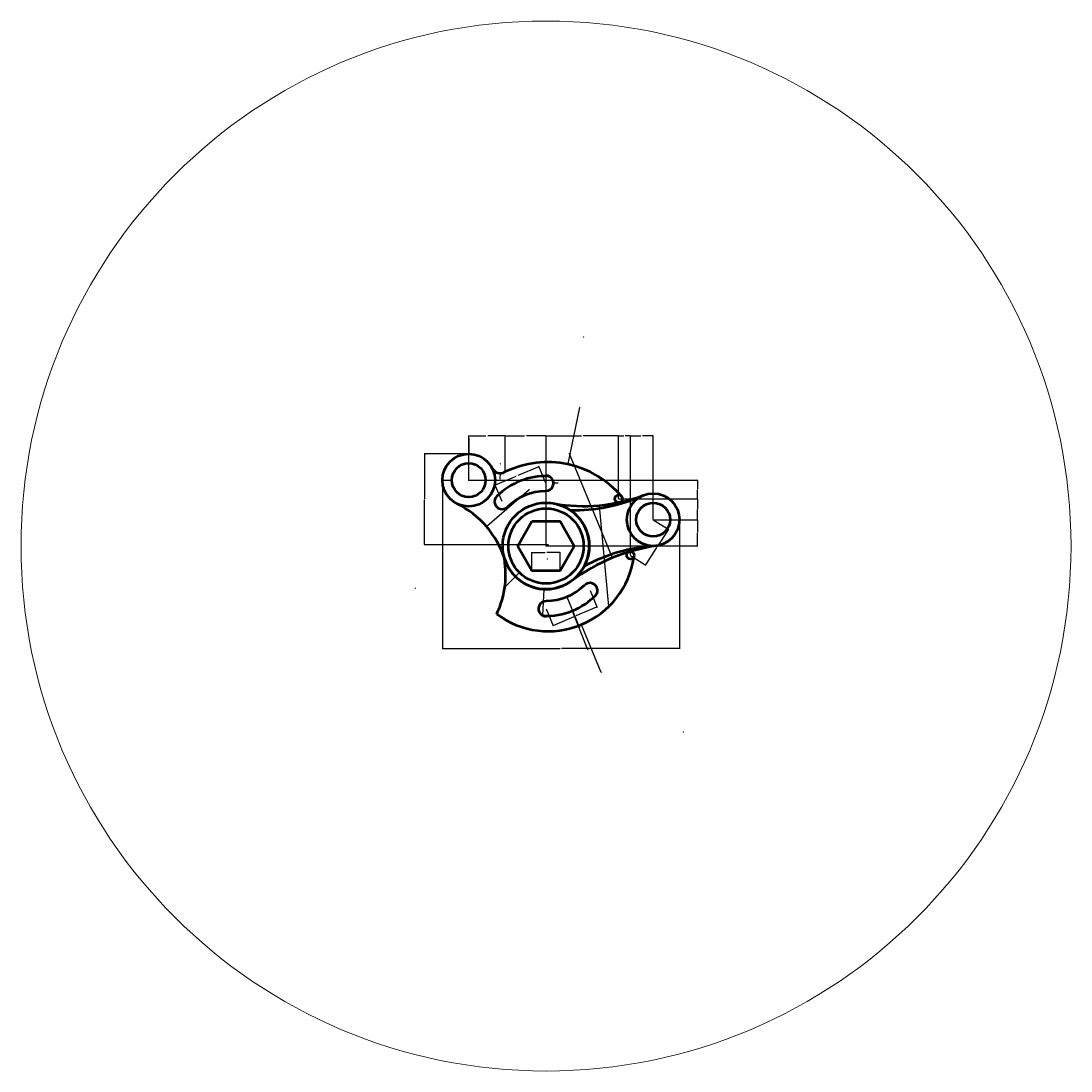
# Model space of a CAD drawing. Units: inches. Extents: x -150 to 408, y -282 to 276.
import ezdxf

# ---------------------------------------------------------------- set-up
doc = ezdxf.new("R2010")
doc.units = ezdxf.units.IN
doc.header["$MEASUREMENT"] = 0
for name, color, linetype, lineweight in [('M-CONS', 8, 'Continuous', 18), ('M-DIMS', 2, 'Continuous', 18), ('M-OUTL', 7, 'Continuous', 50)]:
    doc.layers.add(name, color=color, linetype=linetype, lineweight=lineweight)
doc.styles.get("Standard").update_dxf_attribs({"font": 'arial.ttf'})
doc.dimstyles.get("Standard").update_dxf_attribs({"dimtxt": 0.18, "dimasz": 0.18, "dimexe": 0.18, "dimexo": 0.0625, "dimgap": 0.09, "dimtad": 0, "dimtih": 1, "dimtoh": 1, "dimdec": 4, "dimzin": 0, "dimdsep": 46, "dimtxsty": 'Standard', "dimcen": 0.09, "dimadec": 0, "dimazin": 0, "dimtfac": 1, "dimtdec": 4, "dimtofl": 0, "dimtmove": 0, "dimatfit": 3, "dimfxl": 1, "dimtolj": 1, "dimtzin": 0, "dimarcsym": 0})

# ---------------------------------------------------------------- blocks, each defined once
blk = doc.blocks.new('MOUNTING-EYE-28-18')
for radius in [14, 9]:
    blk.add_circle((14, 14), radius)
blk = doc.blocks.new('*D2')
at = {"layer": 'Defpoints', "color": 0, "transparency": 16777216}
for p in [(74.15, 32.2), (200.26, 11.19), (200.26, -57.4)]:
    blk.add_point(p, dxfattribs=at)
at = {"layer": 'M-DIMS', "color": 0, "lineweight": -2, "transparency": 16777216}
for p, q in [((74.15, 32.14), (74.15, -57.58)), ((200.26, 11.12), (200.26, -57.58)), ((74.33, -57.4), (136.83, -57.4)), ((200.08, -57.4), (137.57, -57.4))]:
    blk.add_line(p, q, dxfattribs=at)
at = {"layer": 'M-DIMS', "color": 0, "transparency": 16777216}
for points in [[(74.33, -57.37), (74.33, -57.43), (74.15, -57.4)], [(200.08, -57.37), (200.08, -57.43), (200.26, -57.4)]]:
    blk.add_solid(points, dxfattribs=at)
at = {"layer": 'M-DIMS', "color": 0, "transparency": 16777216, "insert": (137.2, -57.4), "char_height": 0.18, "attachment_point": 5}
blk.add_mtext('\\A1;126.1', dxfattribs=at)
blk = doc.blocks.new('*D3')
at = {"layer": 'Defpoints', "color": 0, "transparency": 16777216}
for p in [(88.15, 46.2), (64.55, -2.28), (130.5, -2.28)]:
    blk.add_point(p, dxfattribs=at)
at = {"layer": 'M-DIMS', "color": 0, "lineweight": -2, "transparency": 16777216}
for p, q in [((88.08, 46.2), (64.37, 46.2)), ((64.55, 46.02), (64.55, 22.14)), ((64.55, -2.1), (64.55, 21.78)), ((130.44, -2.28), (64.37, -2.28))]:
    blk.add_line(p, q, dxfattribs=at)
at = {"layer": 'M-DIMS', "color": 0, "transparency": 16777216}
for points in [[(64.52, 46.02), (64.58, 46.02), (64.55, 46.2)], [(64.52, -2.1), (64.58, -2.1), (64.55, -2.28)]]:
    blk.add_solid(points, dxfattribs=at)
at = {"layer": 'M-DIMS', "color": 0, "transparency": 16777216, "insert": (64.55, 21.96), "char_height": 0.18, "attachment_point": 5}
blk.add_mtext('\\A1;48.48', dxfattribs=at)
blk = doc.blocks.new('*D4')
at = {"layer": 'Defpoints', "color": 0, "transparency": 16777216}
for p in [(107.45, 55.8), (107.45, 36.55), (88.15, 32.2)]:
    blk.add_point(p, dxfattribs=at)
at = {"layer": 'M-DIMS', "color": 0, "lineweight": -2, "transparency": 16777216}
for p, q in [((88.15, 32.26), (88.15, 55.98)), ((107.45, 36.61), (107.45, 55.98)), ((88.33, 55.8), (97.34, 55.8)), ((107.27, 55.8), (98.25, 55.8))]:
    blk.add_line(p, q, dxfattribs=at)
at = {"layer": 'M-DIMS', "color": 0, "transparency": 16777216}
for points in [[(88.33, 55.83), (88.33, 55.77), (88.15, 55.8)], [(107.27, 55.83), (107.27, 55.77), (107.45, 55.8)]]:
    blk.add_solid(points, dxfattribs=at)
at = {"layer": 'M-DIMS', "color": 0, "transparency": 16777216, "insert": (97.8, 55.8), "char_height": 0.18, "attachment_point": 5}
blk.add_mtext('\\A1;19.302', dxfattribs=at)
blk = doc.blocks.new('*D5')
at = {"layer": 'Defpoints', "color": 0, "transparency": 16777216}
for p in [(129.26, 55.8), (107.45, 36.55), (129.26, -2.81)]:
    blk.add_point(p, dxfattribs=at)
at = {"layer": 'M-DIMS', "color": 0, "lineweight": -2, "transparency": 16777216}
for p, q in [((107.45, 36.61), (107.45, 55.98)), ((129.26, -2.75), (129.26, 55.98)), ((107.63, 55.8), (117.89, 55.8)), ((129.08, 55.8), (118.82, 55.8))]:
    blk.add_line(p, q, dxfattribs=at)
at = {"layer": 'M-DIMS', "color": 0, "transparency": 16777216}
for points in [[(107.63, 55.83), (107.63, 55.77), (107.45, 55.8)], [(129.08, 55.83), (129.08, 55.77), (129.26, 55.8)]]:
    blk.add_solid(points, dxfattribs=at)
at = {"layer": 'M-DIMS', "color": 0, "transparency": 16777216, "insert": (118.35, 55.8), "char_height": 0.18, "attachment_point": 5}
blk.add_mtext('\\A1;21.808', dxfattribs=at)
blk = doc.blocks.new('*D6')
at = {"layer": 'Defpoints', "color": 0, "transparency": 16777216}
for p in [(167.85, 55.8), (167.85, 22.33), (129.26, -2.81)]:
    blk.add_point(p, dxfattribs=at)
at = {"layer": 'M-DIMS', "color": 0, "lineweight": -2, "transparency": 16777216}
for p, q in [((129.26, -2.75), (129.26, 55.98)), ((167.85, 22.39), (167.85, 55.98)), ((129.44, 55.8), (148.16, 55.8)), ((167.67, 55.8), (148.95, 55.8))]:
    blk.add_line(p, q, dxfattribs=at)
at = {"layer": 'M-DIMS', "color": 0, "transparency": 16777216}
for points in [[(129.44, 55.83), (129.44, 55.77), (129.26, 55.8)], [(167.67, 55.83), (167.67, 55.77), (167.85, 55.8)]]:
    blk.add_solid(points, dxfattribs=at)
at = {"layer": 'M-DIMS', "color": 0, "transparency": 16777216, "insert": (148.55, 55.8), "char_height": 0.18, "attachment_point": 5}
blk.add_mtext('\\A1;38.59', dxfattribs=at)
blk = doc.blocks.new('*D7')
at = {"layer": 'Defpoints', "color": 0, "transparency": 16777216}
for p in [(174.16, 55.8), (167.85, 22.33), (174.16, -7.75)]:
    blk.add_point(p, dxfattribs=at)
at = {"layer": 'M-DIMS', "color": 0, "lineweight": -2, "transparency": 16777216}
for p, q in [((167.85, 22.39), (167.85, 55.98)), ((174.16, -7.68), (174.16, 55.98)), ((168.03, 55.8), (170.61, 55.8)), ((173.98, 55.8), (171.4, 55.8))]:
    blk.add_line(p, q, dxfattribs=at)
at = {"layer": 'M-DIMS', "color": 0, "transparency": 16777216}
for points in [[(168.03, 55.83), (168.03, 55.77), (167.85, 55.8)], [(173.98, 55.83), (173.98, 55.77), (174.16, 55.8)]]:
    blk.add_solid(points, dxfattribs=at)
at = {"layer": 'M-DIMS', "color": 0, "transparency": 16777216, "insert": (171, 55.8), "char_height": 0.18, "attachment_point": 5}
blk.add_mtext('\\A1;6.312', dxfattribs=at)
blk = doc.blocks.new('*D8')
at = {"layer": 'Defpoints', "color": 0, "transparency": 16777216}
for p in [(186.26, 55.8), (186.26, 11.19), (174.16, -7.75)]:
    blk.add_point(p, dxfattribs=at)
at = {"layer": 'M-DIMS', "color": 0, "lineweight": -2, "transparency": 16777216}
for p, q in [((174.16, -7.68), (174.16, 55.98)), ((186.26, 11.25), (186.26, 55.98)), ((174.34, 55.8), (179.75, 55.8)), ((186.08, 55.8), (180.66, 55.8))]:
    blk.add_line(p, q, dxfattribs=at)
at = {"layer": 'M-DIMS', "color": 0, "transparency": 16777216}
for points in [[(174.34, 55.83), (174.34, 55.77), (174.16, 55.8)], [(186.08, 55.83), (186.08, 55.77), (186.26, 55.8)]]:
    blk.add_solid(points, dxfattribs=at)
at = {"layer": 'M-DIMS', "color": 0, "transparency": 16777216, "insert": (180.21, 55.8), "char_height": 0.18, "attachment_point": 5}
blk.add_mtext('\\A1;12.096', dxfattribs=at)
blk = doc.blocks.new('*D9')
at = {"layer": 'Defpoints', "color": 0, "transparency": 16777216}
for p in [(88.15, 32.2), (167.85, 22.33), (209.86, 22.33)]:
    blk.add_point(p, dxfattribs=at)
at = {"layer": 'M-DIMS', "color": 0, "lineweight": -2, "transparency": 16777216}
for p, q in [((88.21, 32.2), (210.04, 32.2)), ((209.86, 32.02), (209.86, 27.45)), ((209.86, 22.51), (209.86, 27.08)), ((167.91, 22.33), (210.04, 22.33))]:
    blk.add_line(p, q, dxfattribs=at)
at = {"layer": 'M-DIMS', "color": 0, "transparency": 16777216}
for points in [[(209.83, 32.02), (209.89, 32.02), (209.86, 32.2)], [(209.83, 22.51), (209.89, 22.51), (209.86, 22.33)]]:
    blk.add_solid(points, dxfattribs=at)
at = {"layer": 'M-DIMS', "color": 0, "transparency": 16777216, "insert": (209.86, 27.26), "char_height": 0.18, "attachment_point": 5}
blk.add_mtext('\\A1;9.87', dxfattribs=at)
blk = doc.blocks.new('*D10')
at = {"layer": 'Defpoints', "color": 0, "transparency": 16777216}
for p in [(167.85, 22.33), (186.26, 11.19), (209.86, 11.19)]:
    blk.add_point(p, dxfattribs=at)
at = {"layer": 'M-DIMS', "color": 0, "lineweight": -2, "transparency": 16777216}
for p, q in [((167.91, 22.33), (210.04, 22.33)), ((209.86, 22.15), (209.86, 16.94)), ((186.32, 11.19), (210.04, 11.19)), ((209.86, 11.37), (209.86, 16.58))]:
    blk.add_line(p, q, dxfattribs=at)
at = {"layer": 'M-DIMS', "color": 0, "transparency": 16777216}
for points in [[(209.83, 22.15), (209.89, 22.15), (209.86, 22.33)], [(209.83, 11.37), (209.89, 11.37), (209.86, 11.19)]]:
    blk.add_solid(points, dxfattribs=at)
at = {"layer": 'M-DIMS', "color": 0, "transparency": 16777216, "insert": (209.86, 16.76), "char_height": 0.18, "attachment_point": 5}
blk.add_mtext('\\A1;11.143', dxfattribs=at)
blk = doc.blocks.new('*D11')
at = {"layer": 'Defpoints', "color": 0, "transparency": 16777216}
for p in [(186.26, 11.19), (209.86, 11.19), (129.26, -2.81)]:
    blk.add_point(p, dxfattribs=at)
at = {"layer": 'M-DIMS', "color": 0, "lineweight": -2, "transparency": 16777216}
for p, q in [((186.32, 11.19), (210.04, 11.19)), ((209.86, 11.01), (209.86, 4.37)), ((209.86, -2.63), (209.86, 4.01)), ((129.32, -2.81), (210.04, -2.81))]:
    blk.add_line(p, q, dxfattribs=at)
at = {"layer": 'M-DIMS', "color": 0, "transparency": 16777216}
for points in [[(209.83, 11.01), (209.89, 11.01), (209.86, 11.19)], [(209.83, -2.63), (209.89, -2.63), (209.86, -2.81)]]:
    blk.add_solid(points, dxfattribs=at)
at = {"layer": 'M-DIMS', "color": 0, "transparency": 16777216, "insert": (209.86, 4.19), "char_height": 0.18, "attachment_point": 5}
blk.add_mtext('\\A1;14', dxfattribs=at)
blk = doc.blocks.new('*D12')
at = {"layer": 'Defpoints', "color": 0, "transparency": 16777216}
for p in [(186.26, 11.19), (174.16, -7.75), (182.25, -12.91)]:
    blk.add_point(p, dxfattribs=at)
at = {"layer": 'M-DIMS', "color": 0, "lineweight": -2, "transparency": 16777216}
for p, q in [((186.31, 11.15), (194.5, 5.92)), ((194.25, 5.87), (188.41, -3.27)), ((182.35, -12.76), (188.18, -3.63)), ((174.21, -7.78), (182.4, -13.01))]:
    blk.add_line(p, q, dxfattribs=at)
at = {"layer": 'M-DIMS', "color": 0, "transparency": 16777216}
for points in [[(194.22, 5.88), (194.27, 5.85), (194.35, 6.02)], [(182.32, -12.75), (182.37, -12.78), (182.25, -12.91)]]:
    blk.add_solid(points, dxfattribs=at)
at = {"layer": 'M-DIMS', "color": 0, "transparency": 16777216, "insert": (188.3, -3.45), "char_height": 0.18, "attachment_point": 5}
blk.add_mtext('\\A1;22.465', dxfattribs=at)
blk = doc.blocks.new('*D13')
at = {"layer": 'Defpoints', "color": 0, "transparency": 16777216}
for p in [(136.76, -6.21), (121.75, -15.81), (136.76, -15.81)]:
    blk.add_point(p, dxfattribs=at)
at = {"layer": 'M-DIMS', "color": 0, "lineweight": -2, "transparency": 16777216}
for p, q in [((121.75, -15.75), (121.75, -6.03)), ((121.93, -6.21), (128.89, -6.21)), ((136.58, -6.21), (129.62, -6.21)), ((136.76, -15.75), (136.76, -6.03))]:
    blk.add_line(p, q, dxfattribs=at)
at = {"layer": 'M-DIMS', "color": 0, "transparency": 16777216}
for points in [[(121.93, -6.18), (121.93, -6.24), (121.75, -6.21)], [(136.58, -6.18), (136.58, -6.24), (136.76, -6.21)]]:
    blk.add_solid(points, dxfattribs=at)
at = {"layer": 'M-DIMS', "color": 0, "transparency": 16777216, "insert": (129.26, -6.21), "char_height": 0.18, "attachment_point": 5}
blk.add_mtext('\\A1;15.01', dxfattribs=at)
blk = doc.blocks.new('*D14')
at = {"layer": 'Defpoints', "color": 0, "transparency": 16777216}
for p in [(125.55, 39.41), (129.26, 30.56), (105.9, 20.79)]:
    blk.add_point(p, dxfattribs=at)
at = {"layer": 'M-DIMS', "color": 0, "lineweight": -2, "transparency": 16777216}
for p, q in [((125.39, 39.34), (114.31, 34.71)), ((129.23, 30.62), (125.48, 39.58)), ((102.36, 29.71), (113.44, 34.35)), ((105.88, 20.84), (102.13, 29.81))]:
    blk.add_line(p, q, dxfattribs=at)
at = {"layer": 'M-DIMS', "color": 0, "transparency": 16777216}
for points in [[(125.37, 39.37), (125.4, 39.32), (125.55, 39.41)], [(102.35, 29.74), (102.37, 29.69), (102.2, 29.64)]]:
    blk.add_solid(points, dxfattribs=at)
at = {"layer": 'M-DIMS', "color": 0, "transparency": 16777216, "insert": (113.87, 34.53), "char_height": 0.18, "attachment_point": 5}
blk.add_mtext('\\A1;25.316', dxfattribs=at)
blk = doc.blocks.new('*D15')
at = {"layer": 'Defpoints', "color": 0, "transparency": 16777216}
for p in [(152.67, -26.48), (129.26, -36.21), (132.94, -45.07)]:
    blk.add_point(p, dxfattribs=at)
at = {"layer": 'M-DIMS', "color": 0, "lineweight": -2, "transparency": 16777216}
for p, q in [((152.69, -26.53), (156.42, -35.51)), ((129.28, -36.27), (133.01, -45.24)), ((156.19, -35.41), (145.09, -40.03)), ((133.11, -45.01), (144.21, -40.39))]:
    blk.add_line(p, q, dxfattribs=at)
at = {"layer": 'M-DIMS', "color": 0, "transparency": 16777216}
for points in [[(156.18, -35.38), (156.2, -35.44), (156.36, -35.34)], [(133.1, -44.98), (133.12, -45.03), (132.94, -45.07)]]:
    blk.add_solid(points, dxfattribs=at)
at = {"layer": 'M-DIMS', "color": 0, "transparency": 16777216, "insert": (144.65, -40.21), "char_height": 0.18, "attachment_point": 5}
blk.add_mtext('\\A1;25.356', dxfattribs=at)
blk = doc.blocks.new('*D16')
at = {"layer": 'Defpoints', "color": 0, "transparency": 16777216}
for p in [(88.15, 46.2), (88.15, 18.2)]:
    blk.add_point(p, dxfattribs=at)
at = {"layer": 'M-DIMS', "color": 0, "lineweight": -2, "transparency": 16777216}
for p, q in [((87.97, 54.6), (88.15, 54.6)), ((88.15, 54.6), (88.15, 46.38)), ((88.06, 32.2), (88.24, 32.2)), ((88.15, 32.11), (88.15, 32.29))]:
    blk.add_line(p, q, dxfattribs=at)
at = {"layer": 'M-DIMS', "color": 0, "transparency": 16777216}
blk.add_solid([(88.18, 46.38), (88.12, 46.38), (88.15, 46.2)], dxfattribs=at)
at = {"layer": 'M-DIMS', "color": 0, "transparency": 16777216, "insert": (87.46, 54.6), "char_height": 0.18, "attachment_point": 5}
blk.add_mtext('\\A1;2X ∅28', dxfattribs=at)
blk = doc.blocks.new('*D17')
at = {"layer": 'Defpoints', "color": 0, "transparency": 16777216}
for p in [(79.15, 32.2), (97.15, 32.2)]:
    blk.add_point(p, dxfattribs=at)
at = {"layer": 'M-DIMS', "color": 0, "lineweight": -2, "transparency": 16777216}
for p, q in [((73.75, 32.2), (78.97, 32.2)), ((88.06, 32.2), (88.24, 32.2)), ((88.15, 32.11), (88.15, 32.29))]:
    blk.add_line(p, q, dxfattribs=at)
at = {"layer": 'M-DIMS', "color": 0, "transparency": 16777216}
blk.add_solid([(78.97, 32.23), (78.97, 32.17), (79.15, 32.2)], dxfattribs=at)
at = {"layer": 'M-DIMS', "color": 0, "transparency": 16777216, "insert": (73.24, 32.2), "char_height": 0.18, "attachment_point": 5}
blk.add_mtext('\\A1;2X ∅18', dxfattribs=at)
blk = doc.blocks.new('*D18')
at = {"layer": 'Defpoints', "color": 0, "transparency": 16777216}
for p in [(130.26, 20.16), (128.26, -25.79)]:
    blk.add_point(p, dxfattribs=at)
at = {"layer": 'M-DIMS', "color": 0, "lineweight": -2, "transparency": 16777216}
for p, q in [((129.17, -2.81), (129.35, -2.81)), ((129.26, -2.9), (129.26, -2.72)), ((127.66, -39.58), (128.25, -25.97)), ((127.48, -39.58), (127.66, -39.58))]:
    blk.add_line(p, q, dxfattribs=at)
at = {"layer": 'M-DIMS', "color": 0, "transparency": 16777216}
blk.add_solid([(128.22, -25.97), (128.28, -25.97), (128.26, -25.79)], dxfattribs=at)
at = {"layer": 'M-DIMS', "color": 0, "transparency": 16777216, "insert": (127.16, -39.58), "char_height": 0.18, "attachment_point": 5}
blk.add_mtext('\\A1;∅46', dxfattribs=at)
blk = doc.blocks.new('*D19')
at = {"layer": 'Defpoints', "color": 0, "transparency": 16777216}
for p in [(143.4, 11.33), (115.11, -16.96)]:
    blk.add_point(p, dxfattribs=at)
at = {"layer": 'M-DIMS', "color": 0, "lineweight": -2, "transparency": 16777216}
for p, q in [((129.17, -2.81), (129.35, -2.81)), ((129.26, -2.9), (129.26, -2.72)), ((106.63, -25.44), (114.99, -17.08)), ((106.45, -25.44), (106.63, -25.44))]:
    blk.add_line(p, q, dxfattribs=at)
at = {"layer": 'M-DIMS', "color": 0, "transparency": 16777216}
blk.add_solid([(114.97, -17.06), (115.01, -17.1), (115.11, -16.96)], dxfattribs=at)
at = {"layer": 'M-DIMS', "color": 0, "transparency": 16777216, "insert": (106.13, -25.44), "char_height": 0.18, "attachment_point": 5}
blk.add_mtext('\\A1;∅40', dxfattribs=at)
blk = doc.blocks.new('*D20')
at = {"layer": 'Defpoints', "color": 0, "transparency": 16777216}
for p in [(164.44, -9.17), (202.46, -101.66)]:
    blk.add_point(p, dxfattribs=at)
at = {"layer": 'M-DIMS', "color": 0, "lineweight": -2, "transparency": 16777216}
for p, q in [((141.44, 46.32), (141.62, 46.32)), ((141.62, 46.32), (164.37, -9)), ((202.37, -101.66), (202.55, -101.66)), ((202.46, -101.75), (202.46, -101.57))]:
    blk.add_line(p, q, dxfattribs=at)
at = {"layer": 'M-DIMS', "color": 0, "transparency": 16777216}
blk.add_solid([(164.4, -8.99), (164.34, -9.01), (164.44, -9.17)], dxfattribs=at)
at = {"layer": 'M-DIMS', "color": 0, "transparency": 16777216, "insert": (141.07, 46.32), "char_height": 0.18, "attachment_point": 5}
blk.add_mtext('\\A1;R100', dxfattribs=at)
blk = doc.blocks.new('*D21')
at = {"layer": 'Defpoints', "color": 0, "transparency": 16777216}
for p in [(149.29, 108.4), (157.61, 18.78)]:
    blk.add_point(p, dxfattribs=at)
at = {"layer": 'M-DIMS', "color": 0, "lineweight": -2, "transparency": 16777216}
for p, q in [((149.2, 108.4), (149.38, 108.4)), ((149.29, 108.31), (149.29, 108.49)), ((162.6, -34.99), (157.63, 18.6)), ((162.78, -34.99), (162.6, -34.99))]:
    blk.add_line(p, q, dxfattribs=at)
at = {"layer": 'M-DIMS', "color": 0, "transparency": 16777216}
blk.add_solid([(157.66, 18.6), (157.6, 18.6), (157.61, 18.78)], dxfattribs=at)
at = {"layer": 'M-DIMS', "color": 0, "transparency": 16777216, "insert": (163.28, -34.99), "char_height": 0.18, "attachment_point": 5}
blk.add_mtext('\\A1;3X R90', dxfattribs=at)
blk = doc.blocks.new('*D22')
at = {"layer": 'Defpoints', "color": 0, "transparency": 16777216}
for p in [(140.74, 40.68), (130.1, -9.69)]:
    blk.add_point(p, dxfattribs=at)
at = {"layer": 'M-DIMS', "color": 0, "lineweight": -2, "transparency": 16777216}
for p, q in [((147.13, 70.91), (140.78, 40.86)), ((147.31, 70.91), (147.13, 70.91)), ((130.01, -9.69), (130.19, -9.69)), ((130.1, -9.78), (130.1, -9.6))]:
    blk.add_line(p, q, dxfattribs=at)
at = {"layer": 'M-DIMS', "color": 0, "transparency": 16777216}
blk.add_solid([(140.75, 40.87), (140.81, 40.85), (140.74, 40.68)], dxfattribs=at)
at = {"layer": 'M-DIMS', "color": 0, "transparency": 16777216, "insert": (147.79, 70.91), "char_height": 0.18, "attachment_point": 5}
blk.add_mtext('\\A1;R51.49', dxfattribs=at)
blk = doc.blocks.new('*D23')
at = {"layer": 'Defpoints', "color": 0, "transparency": 16777216}
for p in [(97.64, 7.48), (59.76, -25.16)]:
    blk.add_point(p, dxfattribs=at)
at = {"layer": 'M-DIMS', "color": 0, "lineweight": -2, "transparency": 16777216}
for p, q in [((120.37, 27.06), (97.78, 7.59)), ((120.55, 27.06), (120.37, 27.06)), ((59.67, -25.16), (59.85, -25.16)), ((59.76, -25.25), (59.76, -25.07))]:
    blk.add_line(p, q, dxfattribs=at)
at = {"layer": 'M-DIMS', "color": 0, "transparency": 16777216}
blk.add_solid([(97.76, 7.62), (97.8, 7.57), (97.64, 7.48)], dxfattribs=at)
at = {"layer": 'M-DIMS', "color": 0, "transparency": 16777216, "insert": (121.05, 27.06), "char_height": 0.18, "attachment_point": 5}
blk.add_mtext('\\A1;2X R50', dxfattribs=at)
blk = doc.blocks.new('*D24')
at = {"layer": 'Defpoints', "color": 0, "transparency": 16777216}
for p in [(130.5, -2.28), (148.11, -44.63)]:
    blk.add_point(p, dxfattribs=at)
at = {"layer": 'M-DIMS', "color": 0, "lineweight": -2, "transparency": 16777216}
for p, q in [((130.41, -2.28), (130.59, -2.28)), ((130.5, -2.37), (130.5, -2.19)), ((158.68, -70.04), (148.18, -44.8)), ((158.86, -70.04), (158.68, -70.04))]:
    blk.add_line(p, q, dxfattribs=at)
at = {"layer": 'M-DIMS', "color": 0, "transparency": 16777216}
blk.add_solid([(148.21, -44.78), (148.16, -44.81), (148.11, -44.63)], dxfattribs=at)
at = {"layer": 'M-DIMS', "color": 0, "transparency": 16777216, "insert": (159.34, -70.04), "char_height": 0.18, "attachment_point": 5}
blk.add_mtext('\\A1;R45.86', dxfattribs=at)
blk = doc.blocks.new('*D25')
at = {"layer": 'Defpoints', "color": 0, "transparency": 16777216}
for p in [(129.26, -2.81), (143.2, -37.3)]:
    blk.add_point(p, dxfattribs=at)
at = {"layer": 'M-DIMS', "color": 0, "lineweight": -2, "transparency": 16777216}
for p, q in [((129.17, -2.81), (129.35, -2.81)), ((129.26, -2.9), (129.26, -2.72)), ((151.57, -58), (143.27, -37.47)), ((151.75, -58), (151.57, -58))]:
    blk.add_line(p, q, dxfattribs=at)
at = {"layer": 'M-DIMS', "color": 0, "transparency": 16777216}
blk.add_solid([(143.3, -37.46), (143.24, -37.48), (143.2, -37.3)], dxfattribs=at)
at = {"layer": 'M-DIMS', "color": 0, "transparency": 16777216, "insert": (152.36, -58), "char_height": 0.18, "attachment_point": 5}
blk.add_mtext('\\A1;2X R37.2', dxfattribs=at)
blk = doc.blocks.new('*D26')
at = {"layer": 'Defpoints', "color": 0, "transparency": 16777216}
for p in [(129.26, -2.81), (140.36, -29.82)]:
    blk.add_point(p, dxfattribs=at)
at = {"layer": 'M-DIMS', "color": 0, "lineweight": -2, "transparency": 16777216}
for p, q in [((129.17, -2.81), (129.35, -2.81)), ((129.26, -2.9), (129.26, -2.72)), ((147.02, -46.03), (140.43, -29.99)), ((147.2, -46.03), (147.02, -46.03))]:
    blk.add_line(p, q, dxfattribs=at)
at = {"layer": 'M-DIMS', "color": 0, "transparency": 16777216}
blk.add_solid([(140.46, -29.98), (140.4, -30), (140.36, -29.82)], dxfattribs=at)
at = {"layer": 'M-DIMS', "color": 0, "transparency": 16777216, "insert": (147.95, -46.03), "char_height": 0.18, "attachment_point": 5}
blk.add_mtext('\\A1;2X R29.203', dxfattribs=at)
blk = doc.blocks.new('*D27')
at = {"layer": 'Defpoints', "color": 0, "transparency": 16777216}
for p in [(105.03, 40.92), (104.98, 35.92)]:
    blk.add_point(p, dxfattribs=at)
at = {"layer": 'M-DIMS', "color": 0, "lineweight": -2, "transparency": 16777216}
for p, q in [((104.94, 40.92), (105.12, 40.92)), ((105.03, 40.83), (105.03, 41.01)), ((104.95, 32.92), (104.98, 35.74)), ((104.77, 32.92), (104.95, 32.92))]:
    blk.add_line(p, q, dxfattribs=at)
at = {"layer": 'M-DIMS', "color": 0, "transparency": 16777216}
blk.add_solid([(104.95, 35.74), (105.01, 35.74), (104.98, 35.92)], dxfattribs=at)
at = {"layer": 'M-DIMS', "color": 0, "transparency": 16777216, "insert": (104.54, 32.92), "char_height": 0.18, "attachment_point": 5}
blk.add_mtext('\\A1;R5', dxfattribs=at)
blk = doc.blocks.new('*D28')
at = {"layer": 'Defpoints', "color": 0, "transparency": 16777216}
for p in [(129.26, 30.56), (133.26, 30.58)]:
    blk.add_point(p, dxfattribs=at)
at = {"layer": 'M-DIMS', "color": 0, "lineweight": -2, "transparency": 16777216}
for p, q in [((129.17, 30.56), (129.35, 30.56)), ((129.26, 30.47), (129.26, 30.65)), ((135.66, 30.59), (133.44, 30.58))]:
    blk.add_line(p, q, dxfattribs=at)
at = {"layer": 'M-DIMS', "color": 0, "transparency": 16777216}
blk.add_solid([(133.44, 30.61), (133.44, 30.55), (133.26, 30.58)], dxfattribs=at)
at = {"layer": 'M-DIMS', "color": 0, "transparency": 16777216, "insert": (136.09, 30.59), "char_height": 0.18, "attachment_point": 5}
blk.add_mtext('\\A1;4X R4', dxfattribs=at)
blk = doc.blocks.new('*D29')
at = {"layer": 'Defpoints', "color": 0, "transparency": 16777216}
for p in [(167.97, 24.33), (167.73, 20.33)]:
    blk.add_point(p, dxfattribs=at)
at = {"layer": 'M-DIMS', "color": 0, "lineweight": -2, "transparency": 16777216}
for p, q in [((167.85, 22.24), (167.85, 22.42)), ((168.04, 25.52), (167.98, 24.5)), ((168.22, 25.52), (168.04, 25.52)), ((167.76, 22.33), (167.94, 22.33))]:
    blk.add_line(p, q, dxfattribs=at)
at = {"layer": 'M-DIMS', "color": 0, "transparency": 16777216}
blk.add_solid([(167.95, 24.51), (168.01, 24.5), (167.97, 24.33)], dxfattribs=at)
at = {"layer": 'M-DIMS', "color": 0, "transparency": 16777216, "insert": (168.66, 25.52), "char_height": 0.18, "attachment_point": 5}
blk.add_mtext('\\A1;2X ∅4', dxfattribs=at)

msp = doc.modelspace()

# ---------------------------------------------------------------- linework, layer by layer
at = {"layer": 'M-CONS'}
msp.add_circle((129.2562, -2.8145), 279.2296, dxfattribs=at)
at = {"layer": 'M-OUTL'}
for p, q in [((129.2562, 26.3889), (129.2562, 26.5577)), ((145.4337, -19.1634), (145.6387, -19.3705)), ((149.797, -23.5729), (149.8565, -23.633)), ((129.2562, -32.0179), (129.2562, -32.21))]:
    msp.add_line(p, q, dxfattribs=at)
msp.add_lwpolyline([(121.7506, 10.1855), (114.2451, -2.8145), (121.7506, -15.8145), (136.7617, -15.8145), (144.2673, -2.8145), (136.7617, 10.1855)], close=True, dxfattribs=at)
for centre, radius in [((167.8488, 22.3288), 2), ((129.2562, -2.8145), 23), ((129.2562, -2.8145), 20), ((174.1606, -7.7453), 2)]:
    msp.add_circle(centre, radius, dxfattribs=at)
for centre, radius, start, end in [((130.0975, -9.6886), 51.4862, 40.033517, 116.097604), ((105.0256, 40.922), 5, 207.328243, 298.987037), ((129.2562, -2.8145), 37.2034, 88.130642, 134.698162), ((129.2562, 30.5577), 4, 270, 107.661927), ((105.9018, 20.7872), 4, 134.698162, 314.698162), ((129.2562, -2.8145), 29.2034, 90, 134.698162), ((149.2924, 108.395), 90, 259.786763, 290.819218), ((143.9637, 106.1979), 90, 268.860175, 293.995111), ((59.7608, -25.1615), 50, 17.825821, 63.671227), ((129.2562, -2.8145), 23, 197.825821, 55.832332), ((202.463, -101.6566), 100, 98.173155, 126.525286), ((192.7934, -92.6088), 90, 93.60386, 118.738796), ((57.7993, -17.745), 50, 334.816382, 11.801836), ((130.501, -2.2831), 45.863, 233.229245, 351.941012), ((129.2562, -2.8145), 29.2034, 270, 314.698162), ((152.67, -26.4763), 4, 302.214527, 134.698162), ((129.2562, -36.21), 4, 90, 288.85509), ((129.2562, -2.8145), 37.2034, 268.008748, 316.029892)]:
    msp.add_arc(centre, radius, start, end, dxfattribs=at)

# ---------------------------------------------------------------- block references
for p in [(74.146, 18.199), (172.256, -2.8148)]:
    msp.add_blockref('MOUNTING-EYE-28-18', p, dxfattribs=at)

# ---------------------------------------------------------------- dimensions: what is measured, and where the dimension line sits
at = {"layer": 'M-DIMS'}
for center, mpoint, text, override, picture, middle in [((149.2924, 108.395), (157.61, 18.7802), '3X <>', {"dimdec": 0, "dimlfac": 1, "dimrnd": 0, "dimzin": 0, "dimdsep": 46, "dimlunit": 2}, '*D21', (163.2786, -34.9887)), ((129.2562, 30.5577), (133.2561, 30.5802), '4X <>', {"dimdec": 0, "dimlfac": 1, "dimrnd": 0, "dimzin": 0, "dimdsep": 46, "dimlunit": 2}, '*D28', (135.6561, 30.5937)), ((59.7608, -25.1615), (97.6402, 7.4751), '2X <>', {"dimdec": 0, "dimlfac": 1, "dimrnd": 0, "dimzin": 0, "dimdsep": 46, "dimlunit": 2}, '*D23', (121.0474, 27.0572)), ((129.2562, -2.8145), (143.2041, -37.3043), '2X <>', {"dimdec": 1, "dimlfac": 1, "dimrnd": 0, "dimzin": 0, "dimdsep": 46, "dimlunit": 2}, '*D25', (152.3568, -57.9982)), ((129.2562, -2.8145), (140.361, -29.8241), '2X <>', {"dimdec": 3, "dimlfac": 1, "dimrnd": 0, "dimzin": 0, "dimdsep": 46, "dimlunit": 2}, '*D26', (147.9486, -46.0299))]:
    dim = msp.add_radius_dim(center=center, mpoint=mpoint, text=text, dimstyle='Standard', override=override, dxfattribs=at)
    dim.commit()
    dim.dimension.update_dxf_attribs({"geometry": picture, "text_midpoint": middle, "dimtype": 164})
for center, mpoint, override, picture, middle in [((130.0975, -9.6886), (140.744, 40.6848), {"dimdec": 2, "dimlfac": 1, "dimrnd": 0, "dimzin": 0, "dimdsep": 46, "dimlunit": 2}, '*D22', (147.7918, 70.9089)), ((202.463, -101.6566), (164.4381, -9.1682), {"dimdec": 0, "dimlfac": 1, "dimrnd": 0, "dimzin": 0, "dimdsep": 46, "dimlunit": 2}, '*D20', (141.0684, 46.3249)), ((105.0256, 40.922), (104.9798, 35.9222), {"dimdec": 0, "dimlfac": 1, "dimrnd": 0, "dimzin": 0, "dimdsep": 46, "dimlunit": 2}, '*D27', (104.5366, 32.9223)), ((130.501, -2.2831), (148.1149, -44.6288), {"dimdec": 2, "dimlfac": 1, "dimrnd": 0, "dimzin": 0, "dimdsep": 46, "dimlunit": 2}, '*D24', (159.343, -70.0363))]:
    dim = msp.add_radius_dim(center=center, mpoint=mpoint, dimstyle='Standard', override=override, dxfattribs=at)
    dim.commit()
    dim.dimension.update_dxf_attribs({"geometry": picture, "text_midpoint": middle, "dimtype": 164})
for base, p1, p2, override, picture, middle in [((107.4486, 55.7993), (88.1462, 32.1993), (107.4486, 36.5484), {"dimdec": 3, "dimlfac": 1, "dimrnd": 0, "dimzin": 0, "dimdsep": 46, "dimlunit": 2}, '*D4', (97.7974, 55.7993)), ((129.2562, 55.7993), (107.4486, 36.5484), (129.2562, -2.8145), {"dimdec": 3, "dimlfac": 1, "dimrnd": 0, "dimzin": 0, "dimdsep": 46, "dimlunit": 2}, '*D5', (118.3524, 55.7993)), ((167.8488, 55.7993), (129.2562, -2.8145), (167.8488, 22.3288), {"dimdec": 2, "dimlfac": 1, "dimrnd": 0, "dimzin": 0, "dimdsep": 46, "dimlunit": 2}, '*D6', (148.5525, 55.7993)), ((174.1606, 55.7993), (167.8488, 22.3288), (174.1606, -7.7453), {"dimdec": 3, "dimlfac": 1, "dimrnd": 0, "dimzin": 0, "dimdsep": 46, "dimlunit": 2}, '*D7', (171.0047, 55.7993)), ((186.2562, 55.7993), (174.1606, -7.7453), (186.2562, 11.1855), {"dimdec": 3, "dimlfac": 1, "dimrnd": 0, "dimzin": 0, "dimdsep": 46, "dimlunit": 2}, '*D8', (180.2084, 55.7993)), ((200.2562, -57.3951), (74.1462, 32.1993), (200.2562, 11.1855), {"dimdec": 1, "dimlfac": 1, "dimrnd": 0, "dimzin": 0, "dimdsep": 46, "dimlunit": 2}, '*D2', (137.2012, -57.3951)), ((136.7617, -6.2145), (121.7506, -15.8145), (136.7617, -15.8145), {"dimdec": 2, "dimlfac": 1, "dimrnd": 0, "dimzin": 0, "dimdsep": 46, "dimlunit": 2}, '*D13', (129.2562, -6.2145))]:
    dim = msp.add_linear_dim(base=base, p1=p1, p2=p2, dimstyle='Standard', override=override, dxfattribs=at)
    dim.commit()
    dim.dimension.update_dxf_attribs({"geometry": picture, "text_midpoint": middle})
for p1, p2, picture, middle in [((88.1463, 18.1993), (88.146, 46.1993), '*D16', (87.4587, 54.5993)), ((97.1462, 32.1997), (79.1462, 32.199), '*D17', (73.7462, 32.1988)), ((167.7285, 20.3324), (167.9691, 24.3251), '*D29', (168.658, 25.523))]:
    dim = msp.add_diameter_dim_2p(p1=p1, p2=p2, text='2X <>', dimstyle='Standard', override={"dimdec": 0, "dimlfac": 1, "dimrnd": 0, "dimzin": 0, "dimdsep": 46, "dimlunit": 2}, dxfattribs=at)
    dim.commit()
    dim.dimension.update_dxf_attribs({"geometry": picture, "text_midpoint": middle, "dimtype": 163})
for base, p1, p2, angle, override, picture, middle in [((64.5462, -2.2831), (88.1462, 46.1993), (130.501, -2.2831), 90, {"dimdec": 2, "dimlfac": 1, "dimrnd": 0, "dimzin": 0, "dimdsep": 46, "dimlunit": 2}, '*D3', (64.5462, 21.9581)), ((125.5511, 39.4139), (105.9018, 20.7872), (129.2562, 30.5577), 22.702312, {"dimdec": 3, "dimlfac": 1, "dimrnd": 0, "dimzin": 0, "dimdsep": 46, "dimlunit": 2}, '*D14', (113.874, 34.5287)), ((209.8562, 22.3288), (88.1462, 32.1993), (167.8488, 22.3288), 90, {"dimdec": 2, "dimlfac": 1, "dimrnd": 0, "dimzin": 0, "dimdsep": 46, "dimlunit": 2}, '*D9', (209.8562, 27.2641)), ((209.8562, 11.1855), (167.8488, 22.3288), (186.2562, 11.1855), 90, {"dimdec": 3, "dimlfac": 1, "dimrnd": 0, "dimzin": 0, "dimdsep": 46, "dimlunit": 2}, '*D10', (209.8562, 16.7572)), ((209.8562, 11.1855), (129.2562, -2.8145), (186.2562, 11.1855), 90, {"dimdec": 0, "dimlfac": 1, "dimrnd": 0, "dimzin": 0, "dimdsep": 46, "dimlunit": 2}, '*D11', (209.8562, 4.1855)), ((182.2503, -12.9141), (186.2562, 11.1855), (174.1606, -7.7453), 237.424093, {"dimdec": 3, "dimlfac": 1, "dimrnd": 0, "dimzin": 0, "dimdsep": 46, "dimlunit": 2}, '*D12', (188.2981, -3.4487)), ((132.9414, -45.0745), (152.67, -26.4763), (129.2562, -36.21), 202.574075, {"dimdec": 3, "dimlfac": 1, "dimrnd": 0, "dimzin": 0, "dimdsep": 46, "dimlunit": 2}, '*D15', (144.6483, -40.2076))]:
    dim = msp.add_linear_dim(base=base, p1=p1, p2=p2, angle=angle, dimstyle='Standard', override=override, dxfattribs=at)
    dim.commit()
    dim.dimension.update_dxf_attribs({"geometry": picture, "text_midpoint": middle})
for p1, p2, picture, middle in [((130.2564, 20.1638), (128.256, -25.7927), '*D18', (127.1591, -39.5797)), ((143.3986, 11.3273), (115.1137, -16.9563), '*D19', (106.1317, -25.4414))]:
    dim = msp.add_diameter_dim_2p(p1=p1, p2=p2, dimstyle='Standard', override={"dimdec": 0, "dimlfac": 1, "dimrnd": 0, "dimzin": 0, "dimdsep": 46, "dimlunit": 2}, dxfattribs=at)
    dim.commit()
    dim.dimension.update_dxf_attribs({"geometry": picture, "text_midpoint": middle, "dimtype": 163})

doc.saveas('drawing.dxf')
